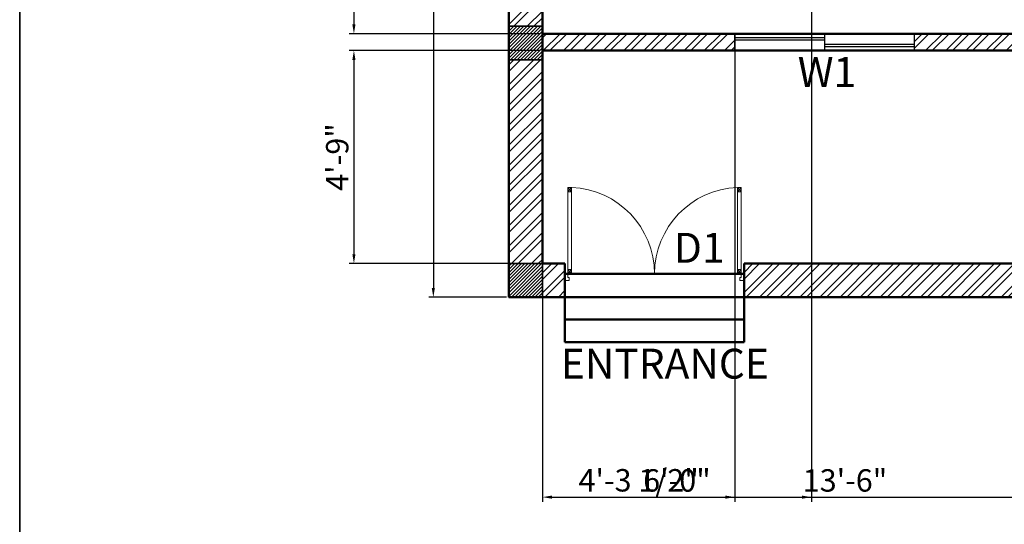
# Model space of a CAD drawing. Units: millimetres. Extents: x 20768 to 23556, y 50760 to 52704.
# Tile 8 of 36: x 20768 to 21032, y 51769 to 51904. Entities that reach past the tile are written whole.
import ezdxf

# ---------------------------------------------------------------- set-up
doc = ezdxf.new("R2010")
doc.units = ezdxf.units.MM
for name, color, linetype, lineweight in [('A-ANNO-DIMS', 2, 'Continuous', 18), ('A-ANNO-TTLB', 7, 'Continuous', 35), ('A-AREA-IDEN', 40, 'Continuous', 18), ('A-FURN', 8, 'Continuous', 18), ('A-GLAZ', 4, 'Continuous', 25), ('A-WALL', 7, 'Continuous', 50), ('A-WALL-PATT', 8, 'Continuous', 13), ('S-ANNO-DIMS', 2, 'Continuous', 18), ('S-COLS', 20, 'Continuous', 35)]:
    doc.layers.add(name, color=color, linetype=linetype, lineweight=lineweight)
doc.styles.get("Standard").update_dxf_attribs({"font": 'arial.ttf'})
doc.dimstyles.new('ISO-25', dxfattribs={"dimtxt": 6, "dimasz": 2.5, "dimexe": 1.25, "dimexo": 0.625, "dimtad": 1, "dimdec": 0, "dimlunit": 3, "dimtxsty": 'Standard', "dimcen": 2.5, "dimadec": 0, "dimazin": 0, "dimtfac": 1, "dimtdec": 0, "dimtmove": 0, "dimatfit": 3, "dimfxl": 1, "dimarcsym": 0})
pattern_1 = [(45, (-81.1113, 0), (-2.69407684, 2.69407684), []), (45, (-79.3152, 0), (-2.69407684, 2.69407684), [])]
pattern_2 = [(45, (-81.11126, 0), (-0.449012806, 0.449012806), [])]

# ---------------------------------------------------------------- blocks, each defined once
blk = doc.blocks.new('md')
for p, q in [((21281.56, 52416.74), (21282.55, 52415.57)), ((21282.55, 52416.74), (21281.56, 52415.57)), ((21282.55, 52415.57), (21281.56, 52415.57)), ((21327.92, 52416.74), (21326.93, 52415.57)), ((21326.93, 52416.74), (21327.92, 52415.57)), ((21326.93, 52415.57), (21327.92, 52415.57)), ((21282.55, 52393.58), (21281.56, 52394.75)), ((21281.56, 52393.58), (21282.55, 52394.75)), ((21282.55, 52394.75), (21281.56, 52394.75)), ((21326.93, 52393.58), (21327.92, 52394.75)), ((21327.92, 52393.58), (21326.93, 52394.75)), ((21326.93, 52394.75), (21327.92, 52394.75))]:
    blk.add_line(p, q)
for points in [[(21281.56, 52393.58), (21281.56, 52416.74), (21282.55, 52416.74), (21282.55, 52393.58)], [(21327.92, 52393.58), (21327.92, 52416.74), (21326.93, 52416.74), (21326.93, 52393.58)], [(21280.74, 52393.58), (21281.56, 52393.58), (21281.56, 52392.59), (21281.86, 52392.59), (21281.86, 52391.84), (21280.74, 52391.84)], [(21328.74, 52393.58), (21327.92, 52393.58), (21327.92, 52392.59), (21327.62, 52392.59), (21327.62, 52391.84), (21328.74, 52391.84)]]:
    blk.add_lwpolyline(points, close=True)
for centre, start, end in [((21281.56, 52393.58), 0, 87.5455), ((21327.92, 52393.58), 92.4545, 180)]:
    blk.add_arc(centre, 23.18, start, end)
blk = doc.blocks.new('*D108')
at = {"layer": 'A-ANNO-DIMS', "color": 0, "lineweight": -2, "transparency": 16777216}
for p, q in [((20898.51, 52522.9), (20877.66, 52522.9)), ((20878.91, 52520.4), (20878.91, 51832.4)), ((20898.51, 51829.9), (20877.66, 51829.9))]:
    blk.add_line(p, q, dxfattribs=at)
at = {"layer": 'A-ANNO-DIMS', "color": 0, "transparency": 16777216}
for points in [[(20878.49, 52520.4), (20879.33, 52520.4), (20878.91, 52522.9)], [(20878.49, 51832.4), (20879.33, 51832.4), (20878.91, 51829.9)]]:
    blk.add_solid(points, dxfattribs=at)
at = {"layer": 'Defpoints', "color": 0, "transparency": 16777216}
for p in [(20899.14, 52522.9), (20878.91, 51829.9), (20899.14, 51829.9)]:
    blk.add_point(p, dxfattribs=at)
at = {"layer": 'A-ANNO-DIMS', "color": 0, "transparency": 16777216, "insert": (20875.22, 52176.4), "char_height": 6, "attachment_point": 5, "rotation": 90}
blk.add_mtext('57\'-9"', dxfattribs=at)
blk = doc.blocks.new('WIN-PLAN-C')
blk.add_line((0, 4.5), (0, 0))
blk.add_lwpolyline([(0, 4.5), (48, 4.5), (48, 0), (0, 0)], close=True)
blk = doc.blocks.new('*D204')
at = {"layer": 'Defpoints', "color": 0, "transparency": 16777216}
for p in [(20908.14, 52080.4), (20857.64, 51900.4), (20908.14, 51900.4)]:
    blk.add_point(p, dxfattribs=at)
at = {"layer": 'S-ANNO-DIMS', "color": 0, "lineweight": -2, "transparency": 16777216}
for p, q in [((20907.51, 52080.4), (20856.39, 52080.4)), ((20857.64, 52077.9), (20857.64, 51902.9)), ((20907.51, 51900.4), (20856.39, 51900.4))]:
    blk.add_line(p, q, dxfattribs=at)
at = {"layer": 'S-ANNO-DIMS', "color": 0, "transparency": 16777216}
for points in [[(20857.22, 52077.9), (20858.06, 52077.9), (20857.64, 52080.4)], [(20857.22, 51902.9), (20858.06, 51902.9), (20857.64, 51900.4)]]:
    blk.add_solid(points, dxfattribs=at)
at = {"layer": 'S-ANNO-DIMS', "color": 0, "transparency": 16777216, "insert": (20853.95, 51990.4), "char_height": 6, "attachment_point": 5, "rotation": 90}
blk.add_mtext('15\'-0"', dxfattribs=at)
blk = doc.blocks.new('*D205')
at = {"layer": 'Defpoints', "color": 0, "transparency": 16777216}
for p in [(20908.14, 51895.9), (20857.64, 51838.9), (20908.14, 51838.9)]:
    blk.add_point(p, dxfattribs=at)
at = {"layer": 'S-ANNO-DIMS', "color": 0, "lineweight": -2, "transparency": 16777216}
for p, q in [((20907.51, 51895.9), (20856.39, 51895.9)), ((20857.64, 51893.4), (20857.64, 51841.4)), ((20907.51, 51838.9), (20856.39, 51838.9))]:
    blk.add_line(p, q, dxfattribs=at)
at = {"layer": 'S-ANNO-DIMS', "color": 0, "transparency": 16777216}
for points in [[(20857.22, 51893.4), (20858.06, 51893.4), (20857.64, 51895.9)], [(20857.22, 51841.4), (20858.06, 51841.4), (20857.64, 51838.9)]]:
    blk.add_solid(points, dxfattribs=at)
at = {"layer": 'S-ANNO-DIMS', "color": 0, "transparency": 16777216, "insert": (20853.95, 51867.4), "char_height": 6, "attachment_point": 5, "rotation": 90}
blk.add_mtext('4\'-9"', dxfattribs=at)
blk = doc.blocks.new('*D206')
at = {"layer": 'Defpoints', "color": 0, "transparency": 16777216}
for p in [(20908.14, 52144.9), (20980.14, 52144.9), (20980.14, 51776.4)]:
    blk.add_point(p, dxfattribs=at)
at = {"layer": 'S-ANNO-DIMS', "color": 0, "lineweight": -2, "transparency": 16777216}
for p, q in [((20908.14, 52144.27), (20908.14, 51775.15)), ((20980.14, 52144.27), (20980.14, 51775.15)), ((20910.64, 51776.4), (20977.64, 51776.4))]:
    blk.add_line(p, q, dxfattribs=at)
at = {"layer": 'S-ANNO-DIMS', "color": 0, "transparency": 16777216}
for points in [[(20910.64, 51776.81), (20910.64, 51775.98), (20908.14, 51776.4)], [(20977.64, 51776.81), (20977.64, 51775.98), (20980.14, 51776.4)]]:
    blk.add_solid(points, dxfattribs=at)
at = {"layer": 'S-ANNO-DIMS', "color": 0, "transparency": 16777216, "insert": (20944.14, 51780.09), "char_height": 6, "attachment_point": 5}
blk.add_mtext('6\'-0"', dxfattribs=at)
blk = doc.blocks.new('*D207')
at = {"layer": 'Defpoints', "color": 0, "transparency": 16777216}
for p in [(20908.14, 52080.4), (21070.14, 52080.4), (21070.14, 51776.4)]:
    blk.add_point(p, dxfattribs=at)
at = {"layer": 'S-ANNO-DIMS', "color": 0, "lineweight": -2, "transparency": 16777216}
for p, q in [((20908.14, 52079.77), (20908.14, 51775.15)), ((21070.14, 52079.77), (21070.14, 51775.15)), ((20910.64, 51776.4), (21067.64, 51776.4))]:
    blk.add_line(p, q, dxfattribs=at)
at = {"layer": 'S-ANNO-DIMS', "color": 0, "transparency": 16777216}
for points in [[(20910.64, 51776.81), (20910.64, 51775.98), (20908.14, 51776.4)], [(21067.64, 51776.81), (21067.64, 51775.98), (21070.14, 51776.4)]]:
    blk.add_solid(points, dxfattribs=at)
at = {"layer": 'S-ANNO-DIMS', "color": 0, "transparency": 16777216, "insert": (20989.14, 51780.09), "char_height": 6, "attachment_point": 5}
blk.add_mtext('13\'-6"', dxfattribs=at)
blk = doc.blocks.new('*D208')
at = {"layer": 'Defpoints', "color": 0, "transparency": 16777216}
for p in [(20908.14, 51900.4), (20959.64, 51900.4), (20959.64, 51776.4)]:
    blk.add_point(p, dxfattribs=at)
at = {"layer": 'S-ANNO-DIMS', "color": 0, "lineweight": -2, "transparency": 16777216}
for p, q in [((20908.14, 51899.77), (20908.14, 51775.15)), ((20959.64, 51899.77), (20959.64, 51775.15)), ((20910.64, 51776.4), (20957.14, 51776.4))]:
    blk.add_line(p, q, dxfattribs=at)
at = {"layer": 'S-ANNO-DIMS', "color": 0, "transparency": 16777216}
for points in [[(20910.64, 51776.81), (20910.64, 51775.98), (20908.14, 51776.4)], [(20957.14, 51776.81), (20957.14, 51775.98), (20959.64, 51776.4)]]:
    blk.add_solid(points, dxfattribs=at)
at = {"layer": 'S-ANNO-DIMS', "color": 0, "transparency": 16777216, "insert": (20933.89, 51780.13), "char_height": 6, "attachment_point": 5}
blk.add_mtext('4\'-3 1/2"', dxfattribs=at)

msp = doc.modelspace()

# ---------------------------------------------------------------- hatches: boundary and pattern name
at = {"layer": 'A-WALL-PATT'}
h = msp.add_hatch(dxfattribs=at)
h.set_pattern_fill('ANSI32', color=256, scale=0.4)
h.set_pattern_definition(pattern_1)
h.paths.add_polyline_path([(20908.14, 52077.9), (20899.14, 52077.9), (20899.14, 51902.4), (20908.14, 51902.4)])
h = msp.add_hatch(dxfattribs=at)
h.set_pattern_fill('ANSI32', color=256, scale=0.4)
h.set_pattern_definition(pattern_1)
h.paths.add_polyline_path([(21080.64, 51900.4), (21074.64, 51900.4), (21074.64, 52036.5), (21070.14, 52036.5), (21070.14, 51900.4), (21007.64, 51900.4), (21007.64, 51895.9), (21080.64, 51895.9)])
h = msp.add_hatch(dxfattribs=at)
h.set_pattern_fill('ANSI31', color=256, scale=0.2)
h.set_pattern_definition(pattern_2)
h.paths.add_polyline_path([(20908.14, 51902.4), (20899.14, 51902.4), (20899.14, 51893.4), (20908.14, 51893.4)])
h = msp.add_hatch(dxfattribs=at)
h.set_pattern_fill('ANSI32', color=256, scale=0.4)
h.set_pattern_definition(pattern_1)
h.paths.add_polyline_path([(20959.64, 51900.4), (20908.14, 51900.4), (20908.14, 51895.9), (20959.64, 51895.9)])
h = msp.add_hatch(dxfattribs=at)
h.set_pattern_fill('ANSI32', color=256, scale=0.4)
h.set_pattern_definition(pattern_1)
h.paths.add_polyline_path([(20908.14, 51893.4), (20899.14, 51893.4), (20899.14, 51838.9), (20908.14, 51838.9)])
h = msp.add_hatch(dxfattribs=at)
h.set_pattern_fill('ANSI31', color=256, scale=0.2)
h.set_pattern_definition(pattern_2)
h.paths.add_polyline_path([(20908.14, 51838.9), (20899.14, 51838.9), (20899.14, 51829.9), (20908.14, 51829.9)])
h = msp.add_hatch(dxfattribs=at)
h.set_pattern_fill('ANSI32', color=256, scale=0.4)
h.set_pattern_definition(pattern_1)
h.paths.add_polyline_path([(20914.14, 51838.9), (20908.14, 51838.9), (20908.14, 51829.9), (20914.14, 51829.9)])
h = msp.add_hatch(dxfattribs=at)
h.set_pattern_fill('ANSI32', color=256, scale=0.4)
h.set_pattern_definition(pattern_1)
h.paths.add_polyline_path([(21124.14, 51838.9), (20962.14, 51838.9), (20962.14, 51836.13), (20962.14, 51836.13), (20962.14, 51834.4), (20962.14, 51829.9), (21124.14, 51829.9)])

# ---------------------------------------------------------------- linework, layer by layer
at = {"layer": 'A-ANNO-TTLB'}
msp.add_lwpolyline([(20768.14, 52703.98), (23555.8, 52703.98), (23555.8, 51623.53), (20768.14, 51623.53)], close=True, dxfattribs=at)
at = {"layer": 'A-GLAZ'}
for p, q in [((20983.64, 51899.26), (20959.64, 51899.26)), ((20983.64, 51900.4), (20983.64, 51895.9)), ((21007.64, 51900.4), (21007.64, 51895.9)), ((20983.64, 51898.69), (20959.64, 51898.69)), ((20983.64, 51897.57), (21007.64, 51897.57)), ((20983.64, 51896.96), (21007.64, 51896.96))]:
    msp.add_line(p, q, dxfattribs=at)
at = {"layer": 'A-WALL'}
for p, q in [((20899.14, 52522.9), (20899.14, 51829.9)), ((20908.14, 52513.9), (20908.14, 51838.9)), ((20908.14, 51900.4), (21070.14, 51900.4)), ((20908.14, 51895.9), (21080.64, 51895.9)), ((20908.14, 51838.9), (20914.14, 51838.9)), ((20914.14, 51838.9), (20914.14, 51829.9)), ((20962.14, 51838.9), (20962.14, 51829.9)), ((20962.14, 51838.9), (21124.14, 51838.9)), ((20914.14, 51836.13), (20962.14, 51836.13)), ((20899.14, 51829.9), (20914.14, 51829.9)), ((20914.14, 51829.9), (20914.14, 51817.9)), ((20914.14, 51829.9), (20962.14, 51829.9)), ((20962.14, 51829.9), (21133.14, 51829.9)), ((20962.14, 51829.9), (20962.14, 51817.9)), ((20914.14, 51823.9), (20962.14, 51823.9)), ((20914.14, 51817.9), (20962.14, 51817.9))]:
    msp.add_line(p, q, dxfattribs=at)
at = {"layer": 'S-COLS'}
for points in [[(20908.14, 51902.4), (20899.14, 51902.4), (20899.14, 51893.4), (20908.14, 51893.4)], [(20908.14, 51838.9), (20899.14, 51838.9), (20899.14, 51829.9), (20908.14, 51829.9)]]:
    msp.add_lwpolyline(points, close=True, dxfattribs=at)

# ---------------------------------------------------------------- block references
at = {"layer": 'A-FURN'}
msp.add_blockref('md', (-366.6, -557.45), dxfattribs=at)
at = {"layer": 'A-GLAZ'}
msp.add_blockref('WIN-PLAN-C', (20959.64, 51895.9), dxfattribs=at)

# ---------------------------------------------------------------- texts
at = {"layer": 'A-AREA-IDEN', "char_height": 8, "attachment_point": 1}
for s, insert in [('W1', (20976.49, 51894.15)), (' D1', (20940.88, 51847.12)), ('ENTRANCE', (20913.05, 51816.11))]:
    msp.add_mtext_dynamic_manual_height_columns(s, width=27.5349, gutter_width=12.5, heights=[0], dxfattribs=dict(at, insert=insert))

# ---------------------------------------------------------------- dimensions: what is measured, and where the dimension line sits
at = {"layer": 'A-ANNO-DIMS'}
dim = msp.add_linear_dim(base=(20878.91, 51829.9), p1=(20899.14, 52522.9), p2=(20899.14, 51829.9), angle=90, dimstyle='ISO-25', override={"dimclrd": 0, "dimclre": 0, "dimclrt": 0}, dxfattribs=at)
dim.commit()
dim.dimension.update_dxf_attribs({"geometry": '*D108', "text_midpoint": (20875.22, 52176.4)})
at = {"layer": 'S-ANNO-DIMS'}
for base, p1, p2, picture, middle in [((20980.14, 51776.4), (20908.14, 52144.9), (20980.14, 52144.9), '*D206', (20944.14, 51780.09)), ((21070.14, 51776.4), (20908.14, 52080.4), (21070.14, 52080.4), '*D207', (20989.14, 51780.09)), ((20959.64, 51776.4), (20908.14, 51900.4), (20959.64, 51900.4), '*D208', (20933.89, 51780.13))]:
    dim = msp.add_linear_dim(base=base, p1=p1, p2=p2, dimstyle='ISO-25', override={"dimdec": 1, "dimlfac": 1, "dimrnd": 0, "dimzin": 1, "dimdsep": 46, "dimlunit": 4, "dimfrac": 2}, dxfattribs=at)
    dim.commit()
    dim.dimension.update_dxf_attribs({"geometry": picture, "text_midpoint": middle})
for base, p1, p2, picture, middle in [((20857.64, 51900.4), (20908.14, 52080.4), (20908.14, 51900.4), '*D204', (20853.95, 51990.4)), ((20857.64, 51838.9), (20908.14, 51895.9), (20908.14, 51838.9), '*D205', (20853.95, 51867.4))]:
    dim = msp.add_linear_dim(base=base, p1=p1, p2=p2, angle=90, dimstyle='ISO-25', override={"dimdec": 1, "dimlfac": 1, "dimrnd": 0, "dimzin": 1, "dimdsep": 46, "dimlunit": 4, "dimfrac": 2}, dxfattribs=at)
    dim.commit()
    dim.dimension.update_dxf_attribs({"geometry": picture, "text_midpoint": middle})

doc.saveas('drawing.dxf')
